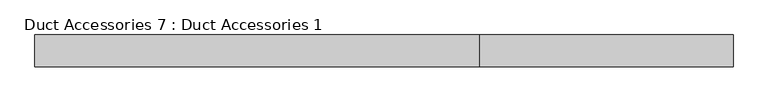
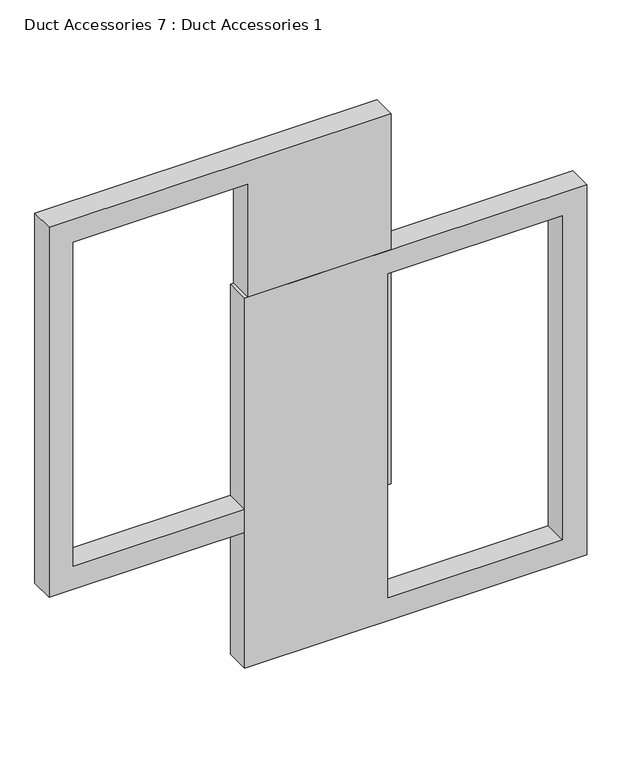
"""IFC4 building model written with IfcOpenShell, lengths in millimetres: damper geometry, Duct Accessories 7 : Duct Accessories 1."""

from ifc_helpers import new_model, si_unit, frame, origin, place, context, project, spatial, polyline, outline, extrude, source, transform, mapped, element, save


def duct_accessories_7_duct_accessories_1_48b7a37f(model_context):
    return source(origin(), model_context, "Body", "SweptSolid", [
        extrude(outline(polyline([(19934.7403114, -12928.36893), (18715.5403114, -12928.36893), (18715.5403114, -11861.56893), (19934.7403114, -11861.56893), (19934.7403114, -12928.36893)]), holes=[polyline([(19858.5403114, -12480.9324751), (19858.5403114, -11937.76893), (18791.7403114, -11937.76893), (18791.7403114, -12480.9324751), (19858.5403114, -12480.9324751)])]), frame((0.0, -447.4934478, 0.0), z_axis=(0.0, 1.0, 0.0), x_axis=(0.0, 0.0, 1.0)), (0.0, 0.0, 1.0), 76.2),
        extrude(outline(polyline([(20382.1767663, -12471.5606701), (20382.1767663, -13538.3606701), (19162.9767663, -13538.3606701), (19162.9767663, -12471.5606701), (20382.1767663, -12471.5606701)]), holes=[polyline([(20305.9767663, -12918.997125), (19239.1767663, -12918.997125), (19239.1767663, -13462.1606701), (20305.9767663, -13462.1606701), (20305.9767663, -12918.997125)])]), frame((0.0, -447.4934478, 0.0), z_axis=(0.0, 1.0, 0.0), x_axis=(0.0, 0.0, 1.0)), (0.0, 0.0, 1.0), 76.2),
    ])


if __name__ == "__main__":
    model = new_model("IFC4")
    model_context = context("Model", 3, world=origin())
    ifc_project = project(units=[si_unit("LENGTHUNIT", "METRE", prefix="MILLI")], contexts=[model_context])
    site = spatial("IfcSite", under=ifc_project)
    building = spatial("IfcBuilding", under=site)
    placement = place(None, origin())
    duct_accessories_7_duct_accessories_1_shape = duct_accessories_7_duct_accessories_1_48b7a37f(model_context)
    element("IfcDamper", 1, ObjectType="Duct Accessories 7 : Duct Accessories 1", at=placement, inside=building, context=model_context, shape_type="MappedRepresentation", body=[
        mapped(duct_accessories_7_duct_accessories_1_shape, transform((0.0, 0.0, 0.0), x_axis=(1.0, 0.0, 0.0), y_axis=(0.0, 1.0, 0.0), z_axis=(0.0, 0.0, 1.0))),
    ])
    save(model, "model.ifc")

# Revit data of these elements
# Element 1 (IfcDamper, "Duct Accessories 7 : Duct Accessories 1")
#   Materials on its faces: "border"
# Materials
#   "border": class "Generic", colour RGB 144 144 144, transparency 0, Cost = 0
